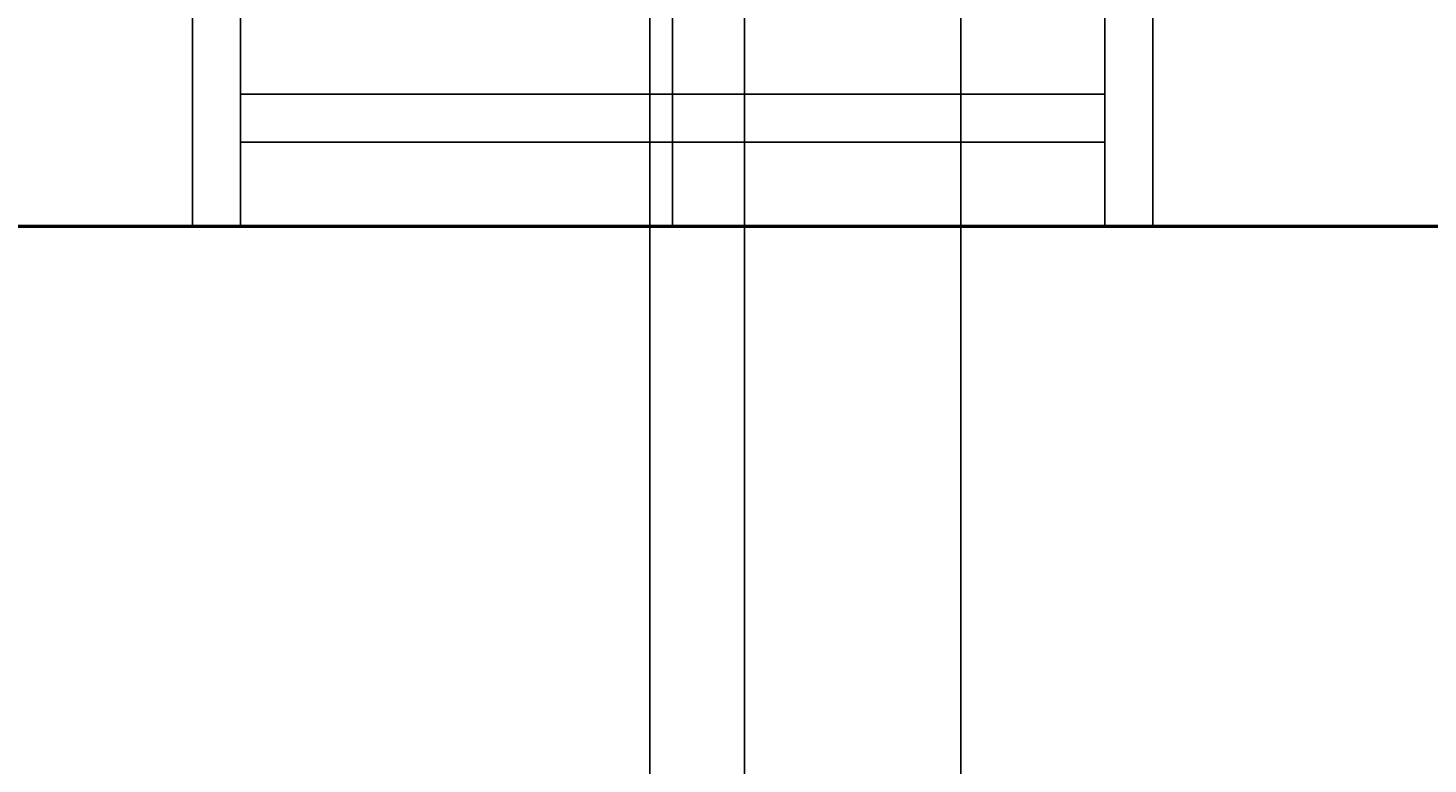
# Model space of a CAD drawing. Units: inches. Extents: x 37 to 824, y -700 to 234.
# Tile 73 of 77: x 332 to 391, y 160 to 190. Entities that reach past the tile are written whole.
import ezdxf

# ---------------------------------------------------------------- set-up
doc = ezdxf.new("R2010")
doc.units = ezdxf.units.IN
doc.header["$MEASUREMENT"] = 0
for name, color, linetype, lineweight in [('A-ANNO-DIMS', 2, 'Continuous', 18), ('A-GLAZ', 4, 'Continuous', 25), ('A-WALL', 2, 'Continuous', 50)]:
    doc.layers.add(name, color=color, linetype=linetype, lineweight=lineweight)
doc.styles.get("Standard").update_dxf_attribs({"font": 'arial.ttf'})
doc.dimstyles.get("Standard").update_dxf_attribs({"dimtxt": 0.18, "dimasz": 0.18, "dimexe": 0.18, "dimexo": 0.0625, "dimgap": 0.09, "dimtad": 0, "dimtih": 1, "dimtoh": 1, "dimdec": 1, "dimzin": 0, "dimdsep": 46, "dimlunit": 4, "dimtxsty": 'Standard', "dimcen": 0.09, "dimadec": 0, "dimazin": 0, "dimtfac": 1, "dimtdec": 1, "dimtofl": 0, "dimtmove": 0, "dimatfit": 3, "dimfxl": 1, "dimtolj": 1, "dimtzin": 0, "dimarcsym": 0})

# ---------------------------------------------------------------- blocks, each defined once
blk = doc.blocks.new('WIN-900')
for p, q in [((0, 9), (0, 0)), ((2, 9), (2, 0)), ((20, 9), (20, 0)), ((38, 9), (38, 0)), ((40, 9), (40, 0)), ((38, 5.5), (2, 5.5)), ((38, 3.5), (2, 3.5))]:
    blk.add_line(p, q)
blk = doc.blocks.new('*D74')
at = {"layer": 'A-ANNO-DIMS', "color": 0, "lineweight": -2, "ltscale": 0.5, "transparency": 16777216}
for p, q in [((371.077, 84.153), (371.077, 234.17)), ((371.257, 233.99), (385.3, 233.99)), ((400.425, 233.99), (386.381, 233.99)), ((400.605, 84.153), (400.605, 234.17))]:
    blk.add_line(p, q, dxfattribs=at)
at = {"layer": 'A-ANNO-DIMS', "color": 0, "ltscale": 0.5, "transparency": 16777216}
for points in [[(371.257, 234.02), (371.257, 233.96), (371.077, 233.99)], [(400.425, 234.02), (400.425, 233.96), (400.605, 233.99)]]:
    blk.add_solid(points, dxfattribs=at)
at = {"layer": 'Defpoints', "color": 0, "ltscale": 0.5, "transparency": 16777216}
for p in [(400.605, 233.99), (371.077, 84.09), (400.605, 84.09)]:
    blk.add_point(p, dxfattribs=at)
at = {"layer": 'A-ANNO-DIMS', "color": 0, "ltscale": 0.5, "transparency": 16777216, "insert": (385.841, 233.99), "char_height": 0.18, "attachment_point": 5}
blk.add_mtext('\\A1;2\'-5 1/2"', dxfattribs=at)
blk = doc.blocks.new('*D78')
at = {"layer": 'A-ANNO-DIMS', "color": 0, "lineweight": -2, "ltscale": 0.5, "transparency": 16777216}
for p, q in [((290.077, 15.153), (290.077, 234.17)), ((290.257, 233.99), (325.747, 233.99)), ((361.897, 233.99), (326.407, 233.99)), ((362.077, 15.153), (362.077, 234.17))]:
    blk.add_line(p, q, dxfattribs=at)
at = {"layer": 'A-ANNO-DIMS', "color": 0, "ltscale": 0.5, "transparency": 16777216}
for points in [[(290.257, 234.02), (290.257, 233.96), (290.077, 233.99)], [(361.897, 234.02), (361.897, 233.96), (362.077, 233.99)]]:
    blk.add_solid(points, dxfattribs=at)
at = {"layer": 'Defpoints', "color": 0, "ltscale": 0.5, "transparency": 16777216}
for p in [(362.077, 233.99), (290.077, 15.09), (362.077, 15.09)]:
    blk.add_point(p, dxfattribs=at)
at = {"layer": 'A-ANNO-DIMS', "color": 0, "ltscale": 0.5, "transparency": 16777216, "insert": (326.077, 233.99), "char_height": 0.18, "attachment_point": 5}
blk.add_mtext('\\A1;6\'-0"', dxfattribs=at)
blk = doc.blocks.new('*D82')
at = {"layer": 'A-ANNO-DIMS', "color": 0, "lineweight": -2, "ltscale": 0.5, "transparency": 16777216}
for p, q in [((299.077, -206.847), (299.077, 234.17)), ((299.257, 233.99), (328.202, 233.99)), ((357.952, 233.99), (329.008, 233.99)), ((358.132, -206.847), (358.132, 234.17))]:
    blk.add_line(p, q, dxfattribs=at)
at = {"layer": 'A-ANNO-DIMS', "color": 0, "ltscale": 0.5, "transparency": 16777216}
for points in [[(299.257, 234.02), (299.257, 233.96), (299.077, 233.99)], [(357.952, 234.02), (357.952, 233.96), (358.132, 233.99)]]:
    blk.add_solid(points, dxfattribs=at)
at = {"layer": 'Defpoints', "color": 0, "ltscale": 0.5, "transparency": 16777216}
for p in [(358.132, 233.99), (299.077, -206.91), (358.132, -206.91)]:
    blk.add_point(p, dxfattribs=at)
at = {"layer": 'A-ANNO-DIMS', "color": 0, "ltscale": 0.5, "transparency": 16777216, "insert": (328.605, 233.99), "char_height": 0.18, "attachment_point": 5}
blk.add_mtext('\\A1;4\'-11"', dxfattribs=at)
blk = doc.blocks.new('*D83')
at = {"layer": 'A-ANNO-DIMS', "color": 0, "lineweight": -2, "ltscale": 0.5, "transparency": 16777216}
for p, q in [((358.132, -206.847), (358.132, 234.17)), ((358.312, 233.99), (388.275, 233.99)), ((418.897, 233.99), (388.934, 233.99)), ((419.077, -206.847), (419.077, 234.17))]:
    blk.add_line(p, q, dxfattribs=at)
at = {"layer": 'A-ANNO-DIMS', "color": 0, "ltscale": 0.5, "transparency": 16777216}
for points in [[(358.312, 234.02), (358.312, 233.96), (358.132, 233.99)], [(418.897, 234.02), (418.897, 233.96), (419.077, 233.99)]]:
    blk.add_solid(points, dxfattribs=at)
at = {"layer": 'Defpoints', "color": 0, "ltscale": 0.5, "transparency": 16777216}
for p in [(419.077, 233.99), (358.132, -206.91), (419.077, -206.91)]:
    blk.add_point(p, dxfattribs=at)
at = {"layer": 'A-ANNO-DIMS', "color": 0, "ltscale": 0.5, "transparency": 16777216, "insert": (388.605, 233.99), "char_height": 0.18, "attachment_point": 5}
blk.add_mtext('\\A1;5\'-1"', dxfattribs=at)

msp = doc.modelspace()

# ---------------------------------------------------------------- linework, layer by layer
at = {"layer": 'A-WALL'}
msp.add_line((299.077, 182.09), (419.077, 182.09), dxfattribs=at)

# ---------------------------------------------------------------- block references
at = {"layer": 'A-GLAZ'}
msp.add_blockref('WIN-900', (339.077, 182.09), dxfattribs=at)

# ---------------------------------------------------------------- dimensions: what is measured, and where the dimension line sits
at = {"layer": 'A-ANNO-DIMS', "ltscale": 0.5}
for base, p1, p2, picture, middle in [((362.077, 233.99), (290.077, 15.09), (362.077, 15.09), '*D78', (326.077, 233.99)), ((358.132, 233.99), (299.077, -206.91), (358.132, -206.91), '*D82', (328.605, 233.99)), ((419.077, 233.99), (358.132, -206.91), (419.077, -206.91), '*D83', (388.605, 233.99)), ((400.605, 233.99), (371.077, 84.09), (400.605, 84.09), '*D74', (385.841, 233.99))]:
    dim = msp.add_linear_dim(base=base, p1=p1, p2=p2, dimstyle='Standard', override={"dimdec": 1, "dimlfac": 1, "dimrnd": 0, "dimzin": 1, "dimdsep": 46, "dimlunit": 4, "dimfrac": 2}, dxfattribs=at)
    dim.commit()
    dim.dimension.update_dxf_attribs({"geometry": picture, "text_midpoint": middle})

doc.saveas('drawing.dxf')
